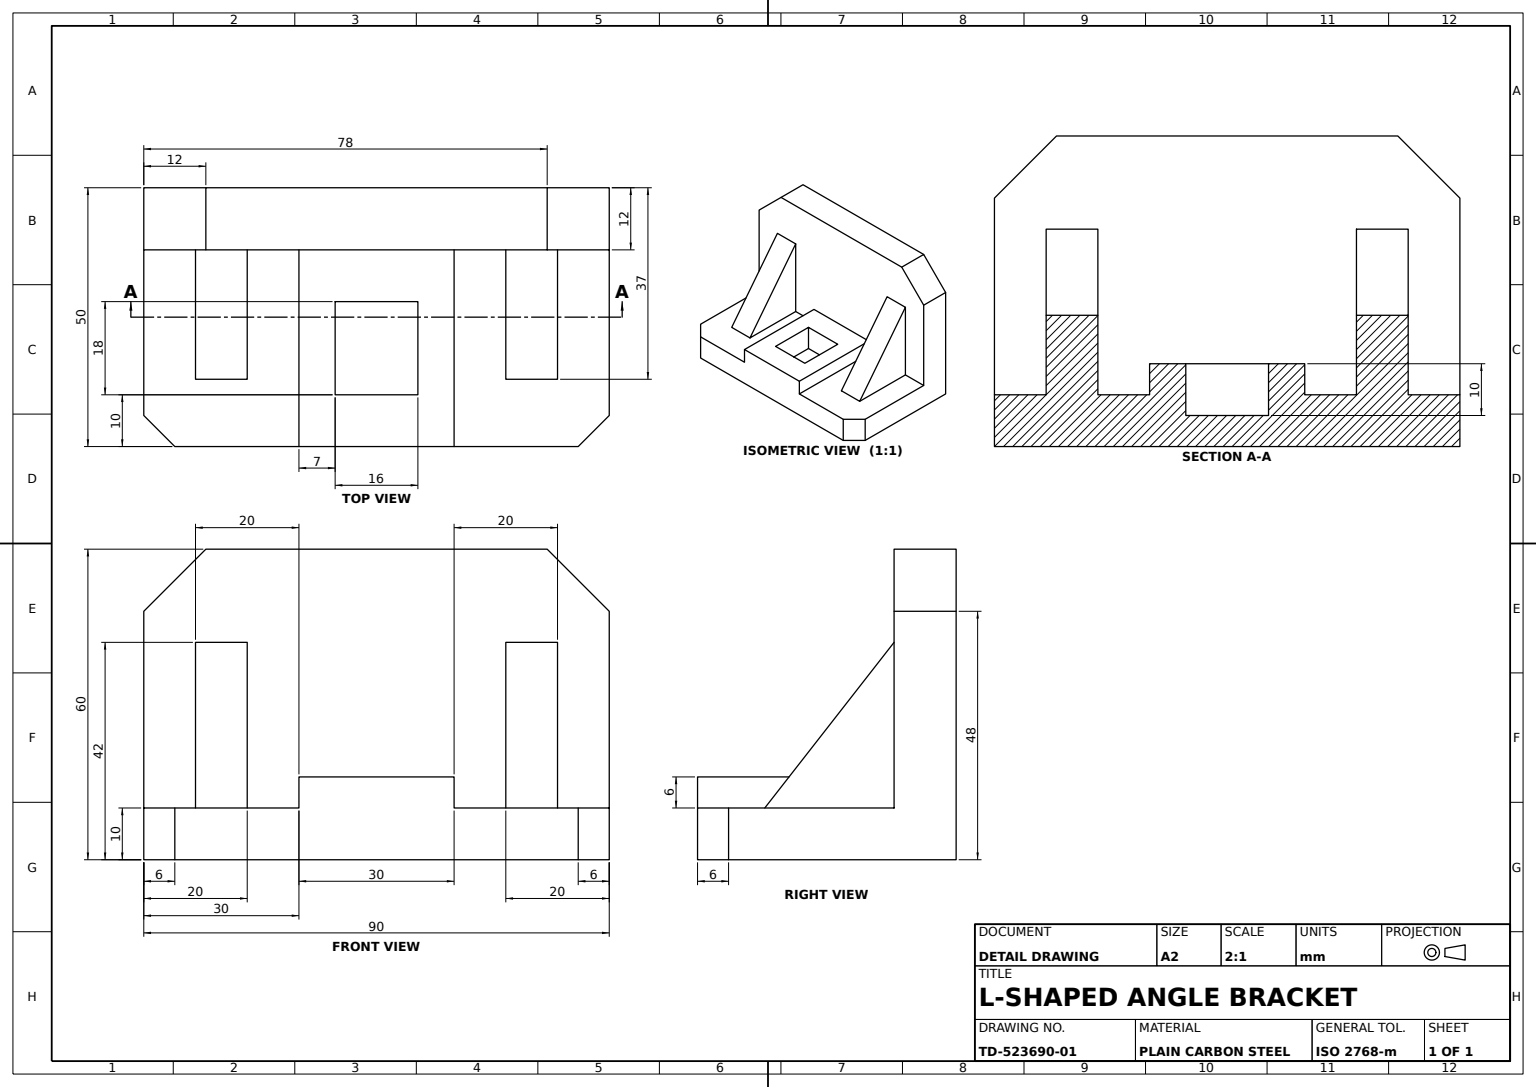
from build123d import *

# Parameters (mm, degrees)
BACK_WALL_DEPTH            = 12
BASE_PLATE_DEPTH           = 10
SQUARE_PAD_PROFILE_30X30_W = 30
SQUARE_PAD_PROFILE_30X30_H = 38
SQUARE_PAD_30X30_DEPTH     = 6
PAD_POCKET_PROFILE_W       = 16
PAD_POCKET_PROFILE_H       = 18
PAD_POCKET_DEPTH           = 10
RIB_1_DEPTH                = 20
RIB_2_DEPTH                = 20
TRIANGULAR_CUT_2_DEPTH     = 10
TRIANGULAR_CUT_1_DEPTH     = 10


with BuildPart() as part:
    # Back Wall Profile → Back Wall (new body)
    with BuildSketch(Plane.XY):
        Polygon((0, 0), (0, 48), (12, 60), (78, 60), (90, 48), (90, 0), align=None)
    extrude(amount=BACK_WALL_DEPTH)

    # Base Plate Profile → Base Plate (add)
    with BuildSketch(Plane.XZ):
        Polygon((90, 12), (0, 12), (0, 44), (6, 50), (84, 50), (90, 44), align=None)
    extrude(amount=-BASE_PLATE_DEPTH)

    # Square Pad Profile 30x30 → Square Pad 30x30 (add)
    with BuildSketch(Plane(origin=(0, 10, 0), x_dir=(1, 0, 0), z_dir=(0, 1, 0))):
        with Locations((45, -31)):
            Rectangle(SQUARE_PAD_PROFILE_30X30_W, SQUARE_PAD_PROFILE_30X30_H)
    extrude(amount=SQUARE_PAD_30X30_DEPTH)

    # Pad Pocket Profile → Pad Pocket (cut)
    with BuildSketch(Plane(origin=(0, 16, 0), x_dir=(1, 0, 0), z_dir=(0, 1, 0))):
        with Locations((45, -31)):
            Rectangle(PAD_POCKET_PROFILE_W, PAD_POCKET_PROFILE_H)
    extrude(amount=-PAD_POCKET_DEPTH, mode=Mode.SUBTRACT)

    # Rib 1 Profile → Rib 1 (add)
    with BuildSketch(Plane.ZY):
        Polygon((12, 10), (12, 42), (37, 10), align=None)
    extrude(amount=-RIB_1_DEPTH)

    # Rib 2 Profile → Rib 2 (add)
    with BuildSketch(Plane(origin=(90, 0, 0), x_dir=(0, 0, -1), z_dir=(1, 0, 0))):
        Polygon((-12, 10), (-12, 42), (-37, 10), align=None)
    extrude(amount=-RIB_2_DEPTH)

    # Triangular Cut 2 Profile → Triangular Cut 2 (cut)
    with BuildSketch(Plane(origin=(90, 0, 0), x_dir=(0, 0, -1), z_dir=(1, 0, 0))):
        Polygon((-12, 42), (-12, 10), (-37, 10), align=None)
    extrude(amount=-TRIANGULAR_CUT_2_DEPTH, mode=Mode.SUBTRACT)

    # Triangular Cut 1 Profile → Triangular Cut 1 (cut)
    with BuildSketch(Plane.ZY):
        Polygon((12, 42), (12, 10), (37, 10), align=None)
    extrude(amount=-TRIANGULAR_CUT_1_DEPTH, mode=Mode.SUBTRACT)


solid = part.part
